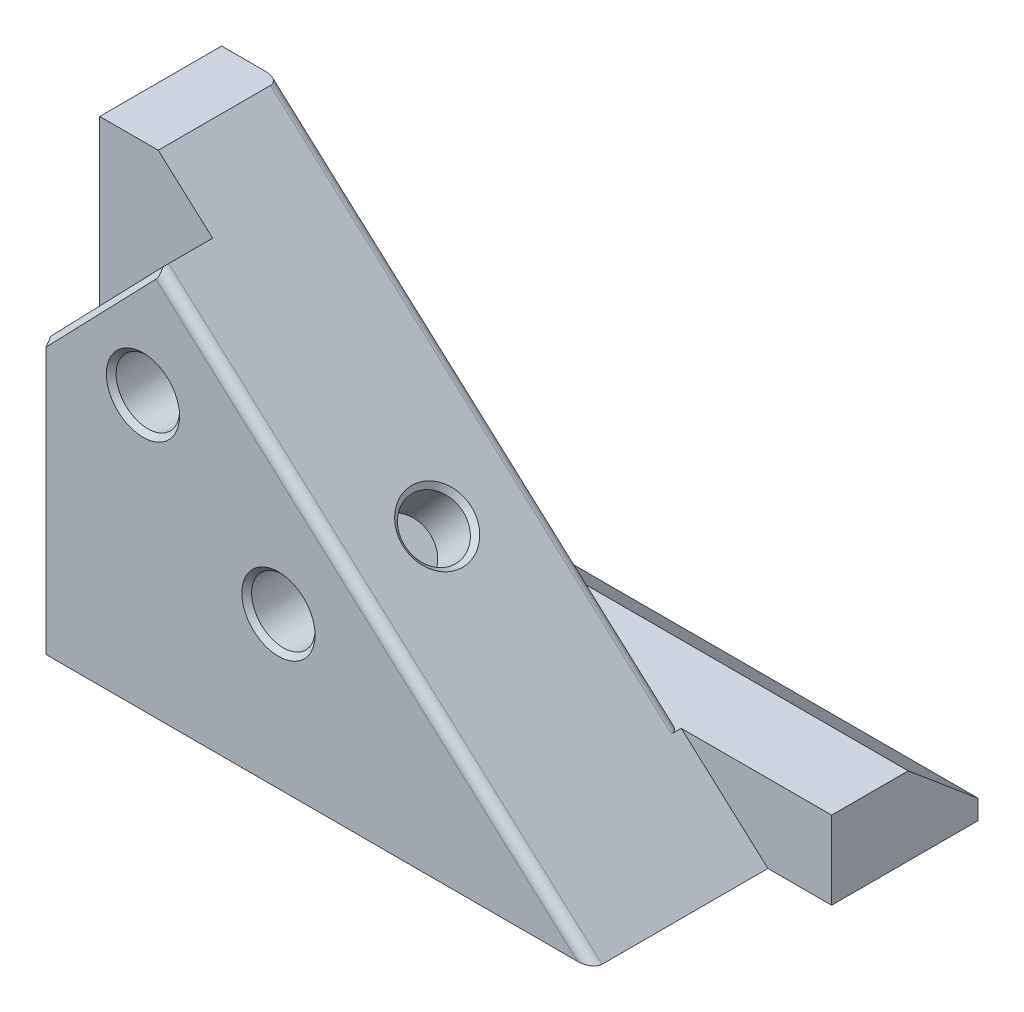
ISO-10303-21;
HEADER;
FILE_DESCRIPTION(('STEP AP214'),'2;1');
FILE_NAME('part.step','',(''),(''),'','','');
FILE_SCHEMA(('AUTOMOTIVE_DESIGN { 1 0 10303 214 1 1 1 1 }'));
ENDSEC;
DATA;
#1=APPLICATION_CONTEXT('core data for automotive mechanical design processes');
#2=APPLICATION_PROTOCOL_DEFINITION('international standard','automotive_design',2000,#1);
#3=PRODUCT_CONTEXT('',#1,'mechanical');
#4=PRODUCT('Part','Part','',(#3));
#5=PRODUCT_RELATED_PRODUCT_CATEGORY('part','',(#4));
#6=PRODUCT_DEFINITION_FORMATION('','',#4);
#7=PRODUCT_DEFINITION_CONTEXT('part definition',#1,'design');
#8=PRODUCT_DEFINITION('design','',#6,#7);
#9=PRODUCT_DEFINITION_SHAPE('','',#8);
#10=(LENGTH_UNIT() NAMED_UNIT(*) SI_UNIT(.MILLI.,.METRE.));
#11=(NAMED_UNIT(*) PLANE_ANGLE_UNIT() SI_UNIT($,.RADIAN.));
#12=(NAMED_UNIT(*) SI_UNIT($,.STERADIAN.) SOLID_ANGLE_UNIT());
#13=UNCERTAINTY_MEASURE_WITH_UNIT(LENGTH_MEASURE(1.E-05),#10,'distance_accuracy_value','');
#14=(GEOMETRIC_REPRESENTATION_CONTEXT(3) GLOBAL_UNCERTAINTY_ASSIGNED_CONTEXT((#13)) GLOBAL_UNIT_ASSIGNED_CONTEXT((#10,
#11,#12)) REPRESENTATION_CONTEXT('',''));
#15=CARTESIAN_POINT('',(0.,0.,0.));
#16=DIRECTION('',(0.,0.,1.));
#17=DIRECTION('',(1.,0.,0.));
#18=AXIS2_PLACEMENT_3D('',#15,#16,#17);
#19=CARTESIAN_POINT('',(0.,90.,18.));
#20=DIRECTION('',(1.,0.,0.));
#21=DIRECTION('',(0.,1.,0.));
#22=AXIS2_PLACEMENT_3D('',#19,#20,#21);
#23=PLANE('',#22);
#24=DIRECTION('',(0.,-1.,0.));
#25=VECTOR('',#24,1.);
#26=CARTESIAN_POINT('',(0.,90.,18.));
#27=LINE('',#26,#25);
#28=CARTESIAN_POINT('',(0.,54.5606472415324,18.));
#29=VERTEX_POINT('',#28);
#30=CARTESIAN_POINT('',(0.,0.,18.));
#31=VERTEX_POINT('',#30);
#32=EDGE_CURVE('E214',#29,#31,#27,.T.);
#33=ORIENTED_EDGE('',*,*,#32,.F.);
#34=DIRECTION('',(0.,0.821249796541805,-0.570568814149568));
#35=VECTOR('',#34,1.);
#36=CARTESIAN_POINT('',(0.,72.1619023724004,5.77140973446541));
#37=LINE('',#36,#35);
#38=CARTESIAN_POINT('',(0.,56.,17.));
#39=VERTEX_POINT('',#38);
#40=EDGE_CURVE('E236',#29,#39,#37,.T.);
#41=ORIENTED_EDGE('',*,*,#40,.T.);
#42=DIRECTION('',(0.,0.,1.));
#43=VECTOR('',#42,1.);
#44=CARTESIAN_POINT('',(0.,56.,7.));
#45=LINE('',#44,#43);
#46=CARTESIAN_POINT('',(0.,56.,7.));
#47=VERTEX_POINT('',#46);
#48=EDGE_CURVE('E202',#47,#39,#45,.T.);
#49=ORIENTED_EDGE('',*,*,#48,.F.);
#50=DIRECTION('',(0.,-1.,0.));
#51=VECTOR('',#50,1.);
#52=CARTESIAN_POINT('',(0.,90.,7.));
#53=LINE('',#52,#51);
#54=CARTESIAN_POINT('',(0.,90.,7.));
#55=VERTEX_POINT('',#54);
#56=EDGE_CURVE('E199',#55,#47,#53,.T.);
#57=ORIENTED_EDGE('',*,*,#56,.F.);
#58=DIRECTION('',(0.,0.,-1.));
#59=VECTOR('',#58,1.);
#60=CARTESIAN_POINT('',(0.,90.,18.));
#61=LINE('',#60,#59);
#62=CARTESIAN_POINT('',(0.,90.,-18.));
#63=VERTEX_POINT('',#62);
#64=EDGE_CURVE('E220',#55,#63,#61,.T.);
#65=ORIENTED_EDGE('',*,*,#64,.T.);
#66=DIRECTION('',(0.,-1.,0.));
#67=VECTOR('',#66,1.);
#68=CARTESIAN_POINT('',(0.,90.,-18.));
#69=LINE('',#68,#67);
#70=CARTESIAN_POINT('',(0.,16.,-18.));
#71=VERTEX_POINT('',#70);
#72=EDGE_CURVE('E206',#63,#71,#69,.T.);
#73=ORIENTED_EDGE('',*,*,#72,.T.);
#74=DIRECTION('',(0.,0.,-1.));
#75=VECTOR('',#74,1.);
#76=CARTESIAN_POINT('',(0.,16.,-18.));
#77=LINE('',#76,#75);
#78=CARTESIAN_POINT('',(0.,16.,-33.6989568888696));
#79=VERTEX_POINT('',#78);
#80=EDGE_CURVE('E181',#71,#79,#77,.T.);
#81=ORIENTED_EDGE('',*,*,#80,.T.);
#82=DIRECTION('',(0.,-0.642787609686543,-0.766044443118975));
#83=VECTOR('',#82,1.);
#84=CARTESIAN_POINT('',(0.,16.,-33.6989568888696));
#85=LINE('',#84,#83);
#86=CARTESIAN_POINT('',(0.,4.,-48.));
#87=VERTEX_POINT('',#86);
#88=EDGE_CURVE('E173',#79,#87,#85,.T.);
#89=ORIENTED_EDGE('',*,*,#88,.T.);
#90=DIRECTION('',(0.,-1.,0.));
#91=VECTOR('',#90,1.);
#92=CARTESIAN_POINT('',(0.,4.,-48.));
#93=LINE('',#92,#91);
#94=CARTESIAN_POINT('',(0.,0.,-48.));
#95=VERTEX_POINT('',#94);
#96=EDGE_CURVE('E167',#87,#95,#93,.T.);
#97=ORIENTED_EDGE('',*,*,#96,.T.);
#98=DIRECTION('',(0.,0.,-1.));
#99=VECTOR('',#98,1.);
#100=CARTESIAN_POINT('',(0.,0.,18.));
#101=LINE('',#100,#99);
#102=EDGE_CURVE('E229',#31,#95,#101,.T.);
#103=ORIENTED_EDGE('',*,*,#102,.F.);
#104=EDGE_LOOP('',(#33,#41,#49,#57,#65,#73,#81,#89,#97,#103));
#105=FACE_BOUND('',#104,.T.);
#106=ADVANCED_FACE('F41',(#105),#23,.F.);
#107=CARTESIAN_POINT('',(0.,0.,18.));
#108=DIRECTION('',(0.,1.,0.));
#109=DIRECTION('',(0.,0.,1.));
#110=AXIS2_PLACEMENT_3D('',#107,#108,#109);
#111=PLANE('',#110);
#112=DIRECTION('',(0.,0.,-1.));
#113=VECTOR('',#112,1.);
#114=CARTESIAN_POINT('',(111.955126334629,0.,18.));
#115=LINE('',#114,#113);
#116=CARTESIAN_POINT('',(111.955126334629,0.,16.));
#117=VERTEX_POINT('',#116);
#118=CARTESIAN_POINT('',(111.955126334629,0.,-18.));
#119=VERTEX_POINT('',#118);
#120=EDGE_CURVE('E226',#117,#119,#115,.T.);
#121=ORIENTED_EDGE('',*,*,#120,.F.);
#122=CARTESIAN_POINT('',(108.966173234899,0.,16.));
#123=DIRECTION('',(0.,1.,0.));
#124=DIRECTION('',(1.,0.,0.));
#125=AXIS2_PLACEMENT_3D('',#122,#123,#124);
#126=ELLIPSE('',#125,2.98895309972924,2.);
#127=CARTESIAN_POINT('',(108.966173234899,0.,18.));
#128=VERTEX_POINT('',#127);
#129=EDGE_CURVE('E11',#117,#128,#126,.F.);
#130=ORIENTED_EDGE('',*,*,#129,.T.);
#131=DIRECTION('',(1.,0.,0.));
#132=VECTOR('',#131,1.);
#133=CARTESIAN_POINT('',(0.,0.,18.));
#134=LINE('',#133,#132);
#135=EDGE_CURVE('E215',#31,#128,#134,.T.);
#136=ORIENTED_EDGE('',*,*,#135,.F.);
#137=ORIENTED_EDGE('',*,*,#102,.T.);
#138=DIRECTION('',(-1.,0.,0.));
#139=VECTOR('',#138,1.);
#140=CARTESIAN_POINT('',(125.,0.,-48.));
#141=LINE('',#140,#139);
#142=CARTESIAN_POINT('',(125.,0.,-48.));
#143=VERTEX_POINT('',#142);
#144=EDGE_CURVE('E189',#143,#95,#141,.T.);
#145=ORIENTED_EDGE('',*,*,#144,.F.);
#146=DIRECTION('',(0.,0.,1.));
#147=VECTOR('',#146,1.);
#148=CARTESIAN_POINT('',(125.,0.,-48.));
#149=LINE('',#148,#147);
#150=CARTESIAN_POINT('',(125.,0.,-18.));
#151=VERTEX_POINT('',#150);
#152=EDGE_CURVE('E152',#143,#151,#149,.T.);
#153=ORIENTED_EDGE('',*,*,#152,.T.);
#154=DIRECTION('',(-1.,0.,0.));
#155=VECTOR('',#154,1.);
#156=CARTESIAN_POINT('',(125.,0.,-18.));
#157=LINE('',#156,#155);
#158=EDGE_CURVE('E169',#151,#119,#157,.T.);
#159=ORIENTED_EDGE('',*,*,#158,.T.);
#160=EDGE_LOOP('',(#121,#130,#136,#137,#145,#153,#159));
#161=FACE_BOUND('',#160,.T.);
#162=ADVANCED_FACE('F298',(#161),#111,.F.);
#163=CARTESIAN_POINT('',(111.955126334629,0.,18.));
#164=DIRECTION('',(-0.669130606358854,-0.743144825477398,0.));
#165=DIRECTION('',(0.743144825477398,-0.669130606358854,0.));
#166=AXIS2_PLACEMENT_3D('',#163,#164,#165);
#167=PLANE('',#166);
#168=CARTESIAN_POINT('',(62.1644230276429,44.8317506260432,0.));
#169=DIRECTION('',(-0.669130606358854,-0.743144825477398,0.));
#170=DIRECTION('',(0.743144825477398,-0.669130606358854,0.));
#171=AXIS2_PLACEMENT_3D('',#168,#169,#170);
#172=CIRCLE('',#171,7.00000000000001);
#173=CARTESIAN_POINT('',(67.3664368059847,40.1478363815312,0.));
#174=VERTEX_POINT('',#173);
#175=EDGE_CURVE('E264',#174,#174,#172,.T.);
#176=ORIENTED_EDGE('',*,*,#175,.T.);
#177=EDGE_LOOP('',(#176));
#178=FACE_BOUND('',#177,.T.);
#179=DIRECTION('',(0.,0.,1.));
#180=VECTOR('',#179,1.);
#181=CARTESIAN_POINT('',(23.147172382161,79.9630409046172,7.));
#182=LINE('',#181,#180);
#183=CARTESIAN_POINT('',(23.147172382161,79.9630409046172,7.));
#184=VERTEX_POINT('',#183);
#185=CARTESIAN_POINT('',(23.147172382161,79.9630409046172,16.));
#186=VERTEX_POINT('',#185);
#187=EDGE_CURVE('E207',#184,#186,#182,.T.);
#188=ORIENTED_EDGE('',*,*,#187,.T.);
#189=DIRECTION('',(-0.743144825477398,0.669130606358854,0.));
#190=VECTOR('',#189,1.);
#191=CARTESIAN_POINT('',(111.955126334629,0.,16.));
#192=LINE('',#191,#190);
#193=EDGE_CURVE('E47',#186,#117,#192,.F.);
#194=ORIENTED_EDGE('',*,*,#193,.T.);
#195=ORIENTED_EDGE('',*,*,#120,.T.);
#196=DIRECTION('',(-0.743144825477398,0.669130606358854,0.));
#197=VECTOR('',#196,1.);
#198=CARTESIAN_POINT('',(111.955126334629,0.,-18.));
#199=LINE('',#198,#197);
#200=CARTESIAN_POINT('',(94.1853260973612,16.,-18.));
#201=VERTEX_POINT('',#200);
#202=EDGE_CURVE('E219',#119,#201,#199,.T.);
#203=ORIENTED_EDGE('',*,*,#202,.T.);
#204=DIRECTION('',(0.,0.,1.));
#205=VECTOR('',#204,1.);
#206=CARTESIAN_POINT('',(94.1853260973612,16.,-18.));
#207=LINE('',#206,#205);
#208=CARTESIAN_POINT('',(94.1853260973612,16.,-16.));
#209=VERTEX_POINT('',#208);
#210=EDGE_CURVE('E146',#201,#209,#207,.T.);
#211=ORIENTED_EDGE('',*,*,#210,.T.);
#212=DIRECTION('',(-0.743144825477398,0.669130606358854,0.));
#213=VECTOR('',#212,1.);
#214=CARTESIAN_POINT('',(111.955126334629,0.,-16.));
#215=LINE('',#214,#213);
#216=CARTESIAN_POINT('',(12.,90.,-16.));
#217=VERTEX_POINT('',#216);
#218=EDGE_CURVE('E268',#209,#217,#215,.T.);
#219=ORIENTED_EDGE('',*,*,#218,.T.);
#220=DIRECTION('',(0.,0.,-1.));
#221=VECTOR('',#220,1.);
#222=CARTESIAN_POINT('',(12.,90.,18.));
#223=LINE('',#222,#221);
#224=CARTESIAN_POINT('',(12.,90.,7.));
#225=VERTEX_POINT('',#224);
#226=EDGE_CURVE('E222',#225,#217,#223,.T.);
#227=ORIENTED_EDGE('',*,*,#226,.F.);
#228=DIRECTION('',(-0.743144825477398,0.669130606358854,0.));
#229=VECTOR('',#228,1.);
#230=CARTESIAN_POINT('',(12.,90.,7.));
#231=LINE('',#230,#229);
#232=EDGE_CURVE('E196',#184,#225,#231,.T.);
#233=ORIENTED_EDGE('',*,*,#232,.F.);
#234=EDGE_LOOP('',(#188,#194,#195,#203,#211,#219,#227,#233));
#235=FACE_BOUND('',#234,.T.);
#236=ADVANCED_FACE('F318',(#178,#235),#167,.F.);
#237=CARTESIAN_POINT('',(12.,90.,18.));
#238=DIRECTION('',(0.,-1.,0.));
#239=DIRECTION('',(0.,0.,-1.));
#240=AXIS2_PLACEMENT_3D('',#237,#238,#239);
#241=PLANE('',#240);
#242=ORIENTED_EDGE('',*,*,#226,.T.);
#243=CARTESIAN_POINT('',(9.01104690027078,90.,-16.));
#244=DIRECTION('',(0.,-1.,0.));
#245=DIRECTION('',(-1.,0.,0.));
#246=AXIS2_PLACEMENT_3D('',#243,#244,#245);
#247=ELLIPSE('',#246,2.98895309972924,2.);
#248=CARTESIAN_POINT('',(9.01104690027079,90.,-18.));
#249=VERTEX_POINT('',#248);
#250=EDGE_CURVE('E275',#217,#249,#247,.F.);
#251=ORIENTED_EDGE('',*,*,#250,.T.);
#252=DIRECTION('',(-1.,0.,0.));
#253=VECTOR('',#252,1.);
#254=CARTESIAN_POINT('',(12.,90.,-18.));
#255=LINE('',#254,#253);
#256=EDGE_CURVE('E213',#249,#63,#255,.T.);
#257=ORIENTED_EDGE('',*,*,#256,.T.);
#258=ORIENTED_EDGE('',*,*,#64,.F.);
#259=DIRECTION('',(-1.,0.,0.));
#260=VECTOR('',#259,1.);
#261=CARTESIAN_POINT('',(0.,90.,7.));
#262=LINE('',#261,#260);
#263=EDGE_CURVE('E197',#225,#55,#262,.T.);
#264=ORIENTED_EDGE('',*,*,#263,.F.);
#265=EDGE_LOOP('',(#242,#251,#257,#258,#264));
#266=FACE_BOUND('',#265,.T.);
#267=ADVANCED_FACE('F322',(#266),#241,.F.);
#268=CARTESIAN_POINT('',(0.,0.,18.));
#269=DIRECTION('',(0.,0.,1.));
#270=DIRECTION('',(1.,0.,0.));
#271=AXIS2_PLACEMENT_3D('',#268,#269,#270);
#272=PLANE('',#271);
#273=CARTESIAN_POINT('',(47.6366073776308,31.,18.));
#274=DIRECTION('',(0.,0.,1.));
#275=DIRECTION('',(1.,0.,0.));
#276=AXIS2_PLACEMENT_3D('',#273,#274,#275);
#277=CIRCLE('',#276,7.49999999999999);
#278=CARTESIAN_POINT('',(55.1366073776308,31.,18.));
#279=VERTEX_POINT('',#278);
#280=EDGE_CURVE('E258',#279,#279,#277,.F.);
#281=ORIENTED_EDGE('',*,*,#280,.T.);
#282=EDGE_LOOP('',(#281));
#283=FACE_BOUND('',#282,.T.);
#284=CARTESIAN_POINT('',(19.8712945069006,56.,18.));
#285=DIRECTION('',(0.,0.,1.));
#286=DIRECTION('',(1.,0.,0.));
#287=AXIS2_PLACEMENT_3D('',#284,#285,#286);
#288=CIRCLE('',#287,7.49999999999999);
#289=CARTESIAN_POINT('',(27.3712945069006,56.,18.));
#290=VERTEX_POINT('',#289);
#291=EDGE_CURVE('E259',#290,#290,#288,.F.);
#292=ORIENTED_EDGE('',*,*,#291,.T.);
#293=EDGE_LOOP('',(#292));
#294=FACE_BOUND('',#293,.T.);
#295=ORIENTED_EDGE('',*,*,#135,.T.);
#296=DIRECTION('',(-0.743144825477398,0.669130606358854,0.));
#297=VECTOR('',#296,1.);
#298=CARTESIAN_POINT('',(22.5525125320393,77.8072095794355,18.));
#299=LINE('',#298,#297);
#300=CARTESIAN_POINT('',(22.500406685115,77.8541258947378,18.));
#301=VERTEX_POINT('',#300);
#302=EDGE_CURVE('E280',#128,#301,#299,.T.);
#303=ORIENTED_EDGE('',*,*,#302,.T.);
#304=DIRECTION('',(-0.694756719030161,-0.719244813232912,0.));
#305=VECTOR('',#304,1.);
#306=CARTESIAN_POINT('',(0.719244813232909,55.3052432809699,18.));
#307=LINE('',#306,#305);
#308=EDGE_CURVE('E234',#301,#29,#307,.T.);
#309=ORIENTED_EDGE('',*,*,#308,.T.);
#310=ORIENTED_EDGE('',*,*,#32,.T.);
#311=EDGE_LOOP('',(#295,#303,#309,#310));
#312=FACE_BOUND('',#311,.T.);
#313=ADVANCED_FACE('F299',(#283,#294,#312),#272,.T.);
#314=CARTESIAN_POINT('',(0.,0.,-18.));
#315=DIRECTION('',(0.,0.,1.));
#316=DIRECTION('',(1.,0.,0.));
#317=AXIS2_PLACEMENT_3D('',#314,#315,#316);
#318=PLANE('',#317);
#319=CARTESIAN_POINT('',(47.6366073776308,31.,-18.));
#320=DIRECTION('',(0.,0.,1.));
#321=DIRECTION('',(1.,0.,0.));
#322=AXIS2_PLACEMENT_3D('',#319,#320,#321);
#323=CIRCLE('',#322,7.49999999999996);
#324=CARTESIAN_POINT('',(55.1366073776307,31.,-18.));
#325=VERTEX_POINT('',#324);
#326=EDGE_CURVE('E250',#325,#325,#323,.T.);
#327=ORIENTED_EDGE('',*,*,#326,.T.);
#328=EDGE_LOOP('',(#327));
#329=FACE_BOUND('',#328,.T.);
#330=CARTESIAN_POINT('',(19.8712945069006,56.,-18.));
#331=DIRECTION('',(0.,0.,1.));
#332=DIRECTION('',(1.,0.,0.));
#333=AXIS2_PLACEMENT_3D('',#330,#331,#332);
#334=CIRCLE('',#333,7.49999999999996);
#335=CARTESIAN_POINT('',(27.3712945069006,56.,-18.));
#336=VERTEX_POINT('',#335);
#337=EDGE_CURVE('E242',#336,#336,#334,.T.);
#338=ORIENTED_EDGE('',*,*,#337,.T.);
#339=EDGE_LOOP('',(#338));
#340=FACE_BOUND('',#339,.T.);
#341=ORIENTED_EDGE('',*,*,#256,.F.);
#342=DIRECTION('',(-0.743144825477398,0.669130606358854,0.));
#343=VECTOR('',#342,1.);
#344=CARTESIAN_POINT('',(48.7880532992486,54.1846225682998,-18.));
#345=LINE('',#344,#343);
#346=CARTESIAN_POINT('',(91.196372997632,16.,-18.));
#347=VERTEX_POINT('',#346);
#348=EDGE_CURVE('E274',#249,#347,#345,.F.);
#349=ORIENTED_EDGE('',*,*,#348,.T.);
#350=DIRECTION('',(-1.,0.,0.));
#351=VECTOR('',#350,1.);
#352=CARTESIAN_POINT('',(125.,16.,-18.));
#353=LINE('',#352,#351);
#354=EDGE_CURVE('E154',#347,#71,#353,.T.);
#355=ORIENTED_EDGE('',*,*,#354,.T.);
#356=ORIENTED_EDGE('',*,*,#72,.F.);
#357=EDGE_LOOP('',(#341,#349,#355,#356));
#358=FACE_BOUND('',#357,.T.);
#359=ADVANCED_FACE('F314',(#329,#340,#358),#318,.F.);
#360=CARTESIAN_POINT('',(23.147172382161,79.9630409046172,7.));
#361=DIRECTION('',(0.719244813232912,-0.694756719030161,0.));
#362=DIRECTION('',(0.694756719030161,0.719244813232912,0.));
#363=AXIS2_PLACEMENT_3D('',#360,#361,#362);
#364=PLANE('',#363);
#365=DIRECTION('',(0.694756719030161,0.719244813232912,0.));
#366=VECTOR('',#365,1.);
#367=CARTESIAN_POINT('',(23.147172382161,79.9630409046172,17.));
#368=LINE('',#367,#366);
#369=CARTESIAN_POINT('',(22.960898516754,79.7702014431697,17.));
#370=VERTEX_POINT('',#369);
#371=EDGE_CURVE('E235',#39,#370,#368,.T.);
#372=ORIENTED_EDGE('',*,*,#371,.T.);
#373=CARTESIAN_POINT('',(21.7568053225189,78.5236675689647,16.));
#374=DIRECTION('',(0.719244813232912,-0.694756719030161,0.));
#375=DIRECTION('',(0.694756719030161,0.719244813232912,0.));
#376=AXIS2_PLACEMENT_3D('',#373,#374,#375);
#377=ELLIPSE('',#376,2.00122866257838,2.);
#378=EDGE_CURVE('E65',#370,#186,#377,.F.);
#379=ORIENTED_EDGE('',*,*,#378,.T.);
#380=ORIENTED_EDGE('',*,*,#187,.F.);
#381=DIRECTION('',(0.694756719030161,0.719244813232911,0.));
#382=VECTOR('',#381,1.);
#383=CARTESIAN_POINT('',(23.147172382161,79.9630409046172,7.));
#384=LINE('',#383,#382);
#385=EDGE_CURVE('E201',#47,#184,#384,.T.);
#386=ORIENTED_EDGE('',*,*,#385,.F.);
#387=ORIENTED_EDGE('',*,*,#48,.T.);
#388=EDGE_LOOP('',(#372,#379,#380,#386,#387));
#389=FACE_BOUND('',#388,.T.);
#390=ADVANCED_FACE('F287',(#389),#364,.F.);
#391=CARTESIAN_POINT('',(0.,0.,6.99999999999999));
#392=DIRECTION('',(0.,0.,-1.));
#393=DIRECTION('',(-1.,0.,0.));
#394=AXIS2_PLACEMENT_3D('',#391,#392,#393);
#395=PLANE('',#394);
#396=ORIENTED_EDGE('',*,*,#232,.T.);
#397=ORIENTED_EDGE('',*,*,#263,.T.);
#398=ORIENTED_EDGE('',*,*,#56,.T.);
#399=ORIENTED_EDGE('',*,*,#385,.T.);
#400=EDGE_LOOP('',(#396,#397,#398,#399));
#401=FACE_BOUND('',#400,.T.);
#402=ADVANCED_FACE('F330',(#401),#395,.F.);
#403=CARTESIAN_POINT('',(54.8039863576955,36.6571575457918,0.));
#404=DIRECTION('',(0.669130606358854,0.743144825477398,0.));
#405=DIRECTION('',(-0.743144825477398,0.669130606358854,0.));
#406=AXIS2_PLACEMENT_3D('',#403,#404,#405);
#407=CYLINDRICAL_SURFACE('',#406,5.99999999999999);
#408=CARTESIAN_POINT('',(61.495292421284,44.0886058005658,0.));
#409=DIRECTION('',(-0.669130606358853,-0.743144825477399,0.));
#410=DIRECTION('',(0.743144825477399,-0.669130606358853,0.));
#411=AXIS2_PLACEMENT_3D('',#408,#409,#410);
#412=CIRCLE('',#411,5.99999999999999);
#413=CARTESIAN_POINT('',(65.9541613741484,40.0738221624127,0.));
#414=VERTEX_POINT('',#413);
#415=EDGE_CURVE('E265',#414,#414,#412,.F.);
#416=ORIENTED_EDGE('',*,*,#415,.T.);
#417=EDGE_LOOP('',(#416));
#418=FACE_BOUND('',#417,.T.);
#419=CARTESIAN_POINT('',(54.8039863576955,36.6571575457918,0.));
#420=DIRECTION('',(0.669130606358854,0.743144825477398,0.));
#421=DIRECTION('',(-0.743144825477398,0.669130606358854,0.));
#422=AXIS2_PLACEMENT_3D('',#419,#420,#421);
#423=CIRCLE('',#422,5.99999999999999);
#424=CARTESIAN_POINT('',(50.3451174048311,40.671941183945,0.));
#425=VERTEX_POINT('',#424);
#426=EDGE_CURVE('E190',#425,#425,#423,.T.);
#427=ORIENTED_EDGE('',*,*,#426,.F.);
#428=EDGE_LOOP('',(#427));
#429=FACE_BOUND('',#428,.T.);
#430=ADVANCED_FACE('F328',(#418,#429),#407,.F.);
#431=CARTESIAN_POINT('',(54.8039863576955,36.6571575457918,0.));
#432=DIRECTION('',(0.669130606358854,0.743144825477398,0.));
#433=DIRECTION('',(-0.743144825477398,0.669130606358854,0.));
#434=AXIS2_PLACEMENT_3D('',#431,#432,#433);
#435=PLANE('',#434);
#436=ORIENTED_EDGE('',*,*,#426,.T.);
#437=EDGE_LOOP('',(#436));
#438=FACE_BOUND('',#437,.T.);
#439=ADVANCED_FACE('F332',(#438),#435,.T.);
#440=CARTESIAN_POINT('',(125.,0.,-18.));
#441=DIRECTION('',(0.,0.,1.));
#442=DIRECTION('',(1.,0.,0.));
#443=AXIS2_PLACEMENT_3D('',#440,#441,#442);
#444=PLANE('',#443);
#445=ORIENTED_EDGE('',*,*,#202,.F.);
#446=ORIENTED_EDGE('',*,*,#158,.F.);
#447=DIRECTION('',(0.,1.,0.));
#448=VECTOR('',#447,1.);
#449=CARTESIAN_POINT('',(125.,0.,-18.));
#450=LINE('',#449,#448);
#451=CARTESIAN_POINT('',(125.,16.,-18.));
#452=VERTEX_POINT('',#451);
#453=EDGE_CURVE('E163',#151,#452,#450,.T.);
#454=ORIENTED_EDGE('',*,*,#453,.T.);
#455=EDGE_CURVE('E142',#452,#201,#353,.T.);
#456=ORIENTED_EDGE('',*,*,#455,.T.);
#457=EDGE_LOOP('',(#445,#446,#454,#456));
#458=FACE_BOUND('',#457,.T.);
#459=ADVANCED_FACE('F170',(#458),#444,.T.);
#460=CARTESIAN_POINT('',(125.,4.,-48.));
#461=DIRECTION('',(0.,0.,-1.));
#462=DIRECTION('',(-1.,0.,0.));
#463=AXIS2_PLACEMENT_3D('',#460,#461,#462);
#464=PLANE('',#463);
#465=ORIENTED_EDGE('',*,*,#96,.F.);
#466=DIRECTION('',(-1.,0.,0.));
#467=VECTOR('',#466,1.);
#468=CARTESIAN_POINT('',(125.,4.,-48.));
#469=LINE('',#468,#467);
#470=CARTESIAN_POINT('',(125.,4.,-48.));
#471=VERTEX_POINT('',#470);
#472=EDGE_CURVE('E194',#471,#87,#469,.T.);
#473=ORIENTED_EDGE('',*,*,#472,.F.);
#474=DIRECTION('',(0.,-1.,0.));
#475=VECTOR('',#474,1.);
#476=CARTESIAN_POINT('',(125.,4.,-48.));
#477=LINE('',#476,#475);
#478=EDGE_CURVE('E180',#471,#143,#477,.T.);
#479=ORIENTED_EDGE('',*,*,#478,.T.);
#480=ORIENTED_EDGE('',*,*,#144,.T.);
#481=EDGE_LOOP('',(#465,#473,#479,#480));
#482=FACE_BOUND('',#481,.T.);
#483=ADVANCED_FACE('F302',(#482),#464,.T.);
#484=CARTESIAN_POINT('',(125.,16.,-33.6989568888696));
#485=DIRECTION('',(0.,0.766044443118975,-0.642787609686543));
#486=DIRECTION('',(0.,0.642787609686543,0.766044443118975));
#487=AXIS2_PLACEMENT_3D('',#484,#485,#486);
#488=PLANE('',#487);
#489=ORIENTED_EDGE('',*,*,#88,.F.);
#490=DIRECTION('',(-1.,0.,0.));
#491=VECTOR('',#490,1.);
#492=CARTESIAN_POINT('',(125.,16.,-33.6989568888696));
#493=LINE('',#492,#491);
#494=CARTESIAN_POINT('',(125.,16.,-33.6989568888696));
#495=VERTEX_POINT('',#494);
#496=EDGE_CURVE('E155',#495,#79,#493,.T.);
#497=ORIENTED_EDGE('',*,*,#496,.F.);
#498=DIRECTION('',(0.,-0.642787609686543,-0.766044443118975));
#499=VECTOR('',#498,1.);
#500=CARTESIAN_POINT('',(125.,16.,-33.6989568888696));
#501=LINE('',#500,#499);
#502=EDGE_CURVE('E164',#495,#471,#501,.T.);
#503=ORIENTED_EDGE('',*,*,#502,.T.);
#504=ORIENTED_EDGE('',*,*,#472,.T.);
#505=EDGE_LOOP('',(#489,#497,#503,#504));
#506=FACE_BOUND('',#505,.T.);
#507=ADVANCED_FACE('F310',(#506),#488,.T.);
#508=CARTESIAN_POINT('',(125.,16.,-18.));
#509=DIRECTION('',(0.,1.,0.));
#510=DIRECTION('',(0.,0.,1.));
#511=AXIS2_PLACEMENT_3D('',#508,#509,#510);
#512=PLANE('',#511);
#513=ORIENTED_EDGE('',*,*,#80,.F.);
#514=ORIENTED_EDGE('',*,*,#354,.F.);
#515=CARTESIAN_POINT('',(91.196372997632,16.,-16.));
#516=DIRECTION('',(0.,1.,0.));
#517=DIRECTION('',(-1.,0.,0.));
#518=AXIS2_PLACEMENT_3D('',#515,#516,#517);
#519=ELLIPSE('',#518,2.98895309972924,2.);
#520=EDGE_CURVE('E279',#347,#209,#519,.F.);
#521=ORIENTED_EDGE('',*,*,#520,.T.);
#522=ORIENTED_EDGE('',*,*,#210,.F.);
#523=ORIENTED_EDGE('',*,*,#455,.F.);
#524=DIRECTION('',(0.,0.,-1.));
#525=VECTOR('',#524,1.);
#526=CARTESIAN_POINT('',(125.,16.,-18.));
#527=LINE('',#526,#525);
#528=EDGE_CURVE('E143',#452,#495,#527,.T.);
#529=ORIENTED_EDGE('',*,*,#528,.T.);
#530=ORIENTED_EDGE('',*,*,#496,.T.);
#531=EDGE_LOOP('',(#513,#514,#521,#522,#523,#529,#530));
#532=FACE_BOUND('',#531,.T.);
#533=ADVANCED_FACE('F144',(#532),#512,.T.);
#534=CARTESIAN_POINT('',(125.,0.,0.));
#535=DIRECTION('',(-1.,0.,0.));
#536=DIRECTION('',(0.,-1.,0.));
#537=AXIS2_PLACEMENT_3D('',#534,#535,#536);
#538=PLANE('',#537);
#539=ORIENTED_EDGE('',*,*,#453,.F.);
#540=ORIENTED_EDGE('',*,*,#152,.F.);
#541=ORIENTED_EDGE('',*,*,#478,.F.);
#542=ORIENTED_EDGE('',*,*,#502,.F.);
#543=ORIENTED_EDGE('',*,*,#528,.F.);
#544=EDGE_LOOP('',(#539,#540,#541,#542,#543));
#545=FACE_BOUND('',#544,.T.);
#546=ADVANCED_FACE('F158',(#545),#538,.F.);
#547=CARTESIAN_POINT('',(19.8712945069006,56.,107.));
#548=DIRECTION('',(0.,0.,-1.));
#549=DIRECTION('',(-1.,0.,0.));
#550=AXIS2_PLACEMENT_3D('',#547,#548,#549);
#551=CYLINDRICAL_SURFACE('',#550,6.5);
#552=CARTESIAN_POINT('',(19.8712945069006,56.,-17.0000000000001));
#553=DIRECTION('',(0.,0.,1.));
#554=DIRECTION('',(1.,0.,0.));
#555=AXIS2_PLACEMENT_3D('',#552,#553,#554);
#556=CIRCLE('',#555,6.5);
#557=CARTESIAN_POINT('',(26.3712945069006,56.,-17.0000000000001));
#558=VERTEX_POINT('',#557);
#559=EDGE_CURVE('E254',#558,#558,#556,.F.);
#560=ORIENTED_EDGE('',*,*,#559,.T.);
#561=EDGE_LOOP('',(#560));
#562=FACE_BOUND('',#561,.T.);
#563=CARTESIAN_POINT('',(19.8712945069006,56.,17.));
#564=DIRECTION('',(0.,0.,1.));
#565=DIRECTION('',(1.,0.,0.));
#566=AXIS2_PLACEMENT_3D('',#563,#564,#565);
#567=CIRCLE('',#566,6.5);
#568=CARTESIAN_POINT('',(26.3712945069006,56.,17.));
#569=VERTEX_POINT('',#568);
#570=EDGE_CURVE('E249',#569,#569,#567,.T.);
#571=ORIENTED_EDGE('',*,*,#570,.T.);
#572=EDGE_LOOP('',(#571));
#573=FACE_BOUND('',#572,.T.);
#574=ADVANCED_FACE('F477',(#562,#573),#551,.F.);
#575=CARTESIAN_POINT('',(47.6366073776308,31.,107.));
#576=DIRECTION('',(0.,0.,-1.));
#577=DIRECTION('',(-1.,0.,0.));
#578=AXIS2_PLACEMENT_3D('',#575,#576,#577);
#579=CYLINDRICAL_SURFACE('',#578,6.5);
#580=CARTESIAN_POINT('',(47.6366073776308,31.,-17.0000000000001));
#581=DIRECTION('',(0.,0.,1.));
#582=DIRECTION('',(1.,0.,0.));
#583=AXIS2_PLACEMENT_3D('',#580,#581,#582);
#584=CIRCLE('',#583,6.5);
#585=CARTESIAN_POINT('',(54.1366073776308,31.,-17.0000000000001));
#586=VERTEX_POINT('',#585);
#587=EDGE_CURVE('E241',#586,#586,#584,.F.);
#588=ORIENTED_EDGE('',*,*,#587,.T.);
#589=EDGE_LOOP('',(#588));
#590=FACE_BOUND('',#589,.T.);
#591=CARTESIAN_POINT('',(47.6366073776308,31.,17.));
#592=DIRECTION('',(0.,0.,1.));
#593=DIRECTION('',(1.,0.,0.));
#594=AXIS2_PLACEMENT_3D('',#591,#592,#593);
#595=CIRCLE('',#594,6.5);
#596=CARTESIAN_POINT('',(54.1366073776308,31.,17.));
#597=VERTEX_POINT('',#596);
#598=EDGE_CURVE('E238',#597,#597,#595,.T.);
#599=ORIENTED_EDGE('',*,*,#598,.T.);
#600=EDGE_LOOP('',(#599));
#601=FACE_BOUND('',#600,.T.);
#602=ADVANCED_FACE('F358',(#590,#601),#579,.F.);
#603=CARTESIAN_POINT('',(23.147172382161,79.9630409046172,17.));
#604=DIRECTION('',(-0.508582884770242,0.491267187301142,0.70710678118655));
#605=DIRECTION('',(-0.694756719030161,-0.719244813232912,0.));
#606=AXIS2_PLACEMENT_3D('',#603,#604,#605);
#607=PLANE('',#606);
#608=ORIENTED_EDGE('',*,*,#308,.F.);
#609=CARTESIAN_POINT('',(21.0132039599228,79.1932092431916,16.));
#610=DIRECTION('',(-0.508582884770242,0.491267187301142,0.70710678118655));
#611=DIRECTION('',(0.542362071668758,-0.455048799059816,0.706239317575418));
#612=AXIS2_PLACEMENT_3D('',#609,#610,#611);
#613=ELLIPSE('',#612,2.83016471602812,2.);
#614=EDGE_CURVE('E281',#301,#370,#613,.T.);
#615=ORIENTED_EDGE('',*,*,#614,.T.);
#616=ORIENTED_EDGE('',*,*,#371,.F.);
#617=ORIENTED_EDGE('',*,*,#40,.F.);
#618=EDGE_LOOP('',(#608,#615,#616,#617));
#619=FACE_BOUND('',#618,.T.);
#620=ADVANCED_FACE('F289',(#619),#607,.T.);
#621=CARTESIAN_POINT('',(47.6366073776308,31.,-17.0000000000001));
#622=DIRECTION('',(0.,0.,-1.));
#623=DIRECTION('',(-1.,0.,0.));
#624=AXIS2_PLACEMENT_3D('',#621,#622,#623);
#625=CONICAL_SURFACE('',#624,6.5,0.785398163397458);
#626=ORIENTED_EDGE('',*,*,#326,.F.);
#627=EDGE_LOOP('',(#626));
#628=FACE_BOUND('',#627,.T.);
#629=ORIENTED_EDGE('',*,*,#587,.F.);
#630=EDGE_LOOP('',(#629));
#631=FACE_BOUND('',#630,.T.);
#632=ADVANCED_FACE('F352',(#628,#631),#625,.F.);
#633=CARTESIAN_POINT('',(19.8712945069006,56.,-17.0000000000001));
#634=DIRECTION('',(0.,0.,-1.));
#635=DIRECTION('',(-1.,0.,0.));
#636=AXIS2_PLACEMENT_3D('',#633,#634,#635);
#637=CONICAL_SURFACE('',#636,6.5,0.785398163397458);
#638=ORIENTED_EDGE('',*,*,#337,.F.);
#639=EDGE_LOOP('',(#638));
#640=FACE_BOUND('',#639,.T.);
#641=ORIENTED_EDGE('',*,*,#559,.F.);
#642=EDGE_LOOP('',(#641));
#643=FACE_BOUND('',#642,.T.);
#644=ADVANCED_FACE('F365',(#640,#643),#637,.F.);
#645=CARTESIAN_POINT('',(47.6366073776308,31.,17.));
#646=DIRECTION('',(0.,0.,1.));
#647=DIRECTION('',(1.,0.,0.));
#648=AXIS2_PLACEMENT_3D('',#645,#646,#647);
#649=CONICAL_SURFACE('',#648,6.5,0.785398163397458);
#650=ORIENTED_EDGE('',*,*,#280,.F.);
#651=EDGE_LOOP('',(#650));
#652=FACE_BOUND('',#651,.T.);
#653=ORIENTED_EDGE('',*,*,#598,.F.);
#654=EDGE_LOOP('',(#653));
#655=FACE_BOUND('',#654,.T.);
#656=ADVANCED_FACE('F367',(#652,#655),#649,.F.);
#657=CARTESIAN_POINT('',(19.8712945069006,56.,17.));
#658=DIRECTION('',(0.,0.,1.));
#659=DIRECTION('',(1.,0.,0.));
#660=AXIS2_PLACEMENT_3D('',#657,#658,#659);
#661=CONICAL_SURFACE('',#660,6.5,0.785398163397458);
#662=ORIENTED_EDGE('',*,*,#291,.F.);
#663=EDGE_LOOP('',(#662));
#664=FACE_BOUND('',#663,.T.);
#665=ORIENTED_EDGE('',*,*,#570,.F.);
#666=EDGE_LOOP('',(#665));
#667=FACE_BOUND('',#666,.T.);
#668=ADVANCED_FACE('F376',(#664,#667),#661,.F.);
#669=CARTESIAN_POINT('',(61.495292421284,44.0886058005658,0.));
#670=DIRECTION('',(0.669130606358853,0.743144825477399,0.));
#671=DIRECTION('',(-0.743144825477399,0.669130606358853,0.));
#672=AXIS2_PLACEMENT_3D('',#669,#670,#671);
#673=CONICAL_SURFACE('',#672,5.99999999999999,0.785398163397451);
#674=ORIENTED_EDGE('',*,*,#175,.F.);
#675=EDGE_LOOP('',(#674));
#676=FACE_BOUND('',#675,.T.);
#677=ORIENTED_EDGE('',*,*,#415,.F.);
#678=EDGE_LOOP('',(#677));
#679=FACE_BOUND('',#678,.T.);
#680=ADVANCED_FACE('F384',(#676,#679),#673,.F.);
#681=CARTESIAN_POINT('',(110.616865121911,-1.4862896509548,-16.));
#682=DIRECTION('',(-0.743144825477398,0.669130606358854,0.));
#683=DIRECTION('',(-0.669130606358854,-0.743144825477398,0.));
#684=AXIS2_PLACEMENT_3D('',#681,#682,#683);
#685=CYLINDRICAL_SURFACE('',#684,2.);
#686=ORIENTED_EDGE('',*,*,#520,.F.);
#687=ORIENTED_EDGE('',*,*,#348,.F.);
#688=ORIENTED_EDGE('',*,*,#250,.F.);
#689=ORIENTED_EDGE('',*,*,#218,.F.);
#690=EDGE_LOOP('',(#686,#687,#688,#689));
#691=FACE_BOUND('',#690,.T.);
#692=ADVANCED_FACE('F319',(#691),#685,.T.);
#693=CARTESIAN_POINT('',(48.7880532992485,54.1846225682998,16.));
#694=DIRECTION('',(0.743144825477398,-0.669130606358854,0.));
#695=DIRECTION('',(0.669130606358854,0.743144825477398,0.));
#696=AXIS2_PLACEMENT_3D('',#693,#694,#695);
#697=CYLINDRICAL_SURFACE('',#696,2.);
#698=ORIENTED_EDGE('',*,*,#129,.F.);
#699=ORIENTED_EDGE('',*,*,#193,.F.);
#700=ORIENTED_EDGE('',*,*,#378,.F.);
#701=ORIENTED_EDGE('',*,*,#614,.F.);
#702=ORIENTED_EDGE('',*,*,#302,.F.);
#703=EDGE_LOOP('',(#698,#699,#700,#701,#702));
#704=FACE_BOUND('',#703,.T.);
#705=ADVANCED_FACE('F43',(#704),#697,.T.);
#706=CLOSED_SHELL('',(#106,#162,#236,#267,#313,#359,#390,#402,#430,#439,#459,#483,#507,#533,
#546,#574,#602,#620,#632,#644,#656,#668,#680,#692,#705));
#707=MANIFOLD_SOLID_BREP('B2',#706);
#708=ADVANCED_BREP_SHAPE_REPRESENTATION('',(#18,#707),#14);
#709=SHAPE_DEFINITION_REPRESENTATION(#9,#708);
ENDSEC;
END-ISO-10303-21;
